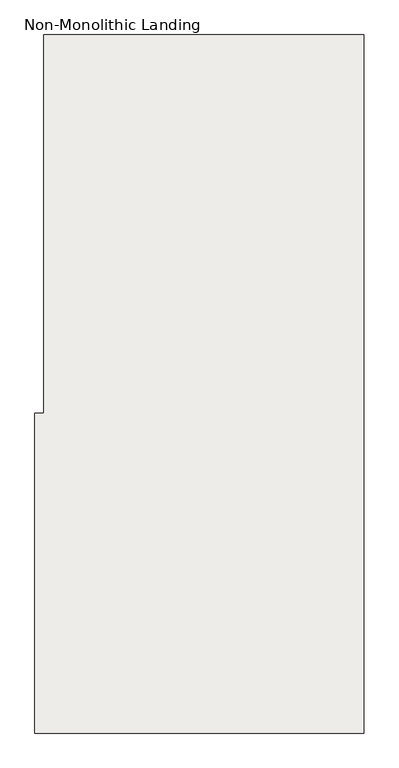
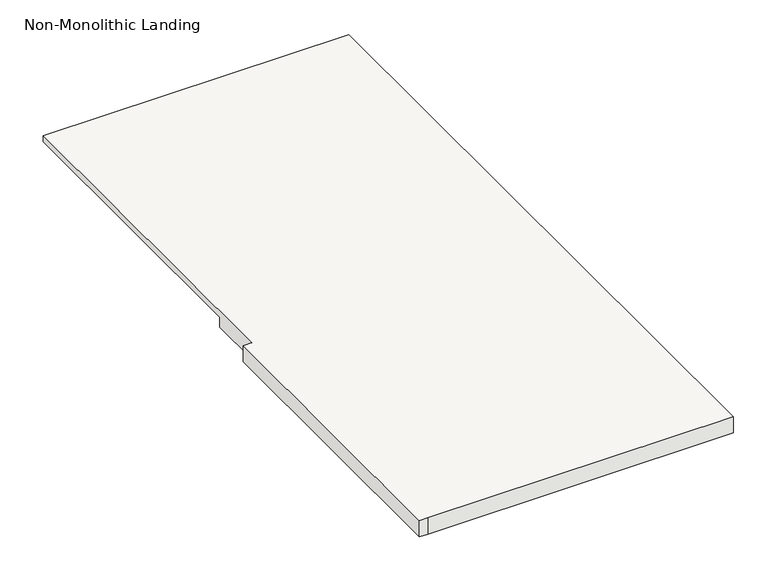
"""IFC4 building model written with IfcOpenShell, lengths in millimetres: slab geometry, Non-Monolithic Landing."""

from ifc_helpers import new_model, si_unit, origin, place, context, project, spatial, faceted_brep, source, transform, mapped, element, save


def non_monolithic_landing_7100f040(model_context):
    return source(origin(), model_context, "Body", "Brep", [
        faceted_brep([(-10706.2571222, 7668.4964313, 1809.75), (-10680.8571222, 7668.4964313, 1784.35), (-10680.8571222, 6754.0964313, 1784.35), (-10706.2571222, 6754.0964313, 1809.75), (-10706.2571222, 6587.3776214, 1828.8), (-10731.6571222, 6587.3776214, 1828.8), (-10731.6571222, 5672.9776214, 1828.8), (-10706.2571222, 5672.9776214, 1828.8), (-9791.8571222, 5672.9776214, 1828.8), (-9791.8571222, 7668.4964313, 1828.8), (-10706.2571222, 7668.4964313, 1828.8), (-10680.8571222, 6754.0964313, 1778.0), (-10680.8571222, 7668.4964313, 1778.0), (-9791.8571222, 7668.4964313, 1778.0), (-9791.8571222, 5672.9776214, 1778.0), (-10706.2571222, 5672.9776214, 1778.0), (-10731.6571222, 5672.9776214, 1778.0), (-10731.6571222, 6587.3776214, 1778.0), (-10706.2571222, 6587.3776214, 1778.0), (-10706.2571222, 6754.0964313, 1778.0)], [[[0, 1, 2, 3]], [[4, 5, 6, 7, 8, 9, 10]], [[11, 12, 13, 14, 15, 16, 17, 18, 19]], [[12, 11, 2, 1]], [[11, 19, 3, 2]], [[4, 10, 0, 3, 19, 18]], [[5, 4, 18, 17]], [[6, 5, 17, 16]], [[7, 6, 16, 15]], [[8, 7, 15, 14]], [[9, 8, 14, 13]], [[10, 9, 13, 12, 1, 0]]]),
    ])


if __name__ == "__main__":
    model = new_model("IFC4")
    model_context = context("Model", 3, world=origin())
    ifc_project = project(units=[si_unit("LENGTHUNIT", "METRE", prefix="MILLI")], contexts=[model_context])
    site = spatial("IfcSite", under=ifc_project)
    building = spatial("IfcBuilding", under=site)
    placement = place(None, origin())
    non_monolithic_landing_shape = non_monolithic_landing_7100f040(model_context)
    element("IfcSlab", 1, ObjectType="Non-Monolithic Landing", at=placement, inside=building, context=model_context, shape_type="MappedRepresentation", body=[
        mapped(non_monolithic_landing_shape, transform((0.0, 0.0, 0.0), x_axis=(1.0, 0.0, 0.0), y_axis=(0.0, 1.0, 0.0), z_axis=(0.0, 0.0, 1.0))),
    ])
    save(model, "model.ifc")
